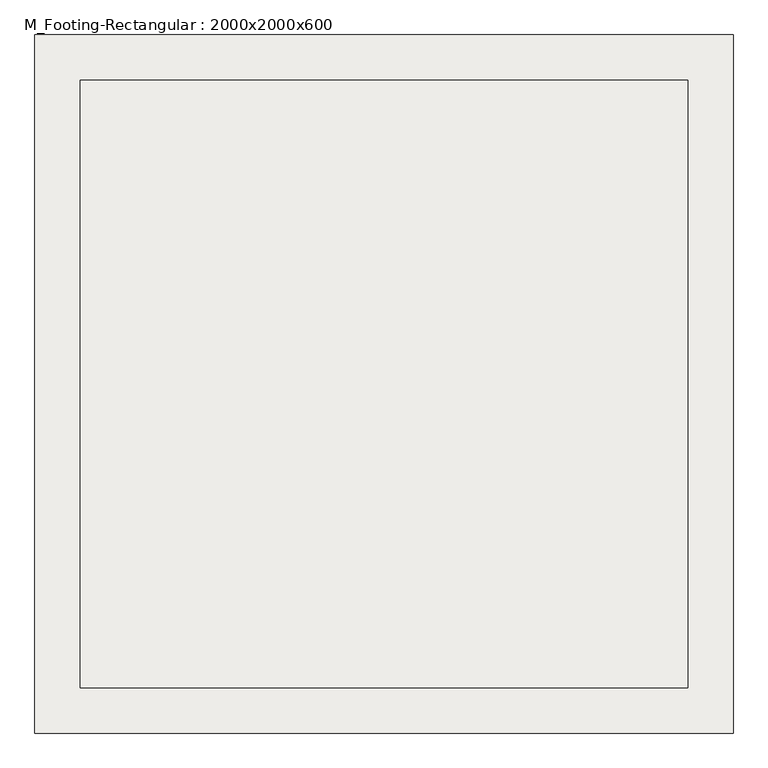
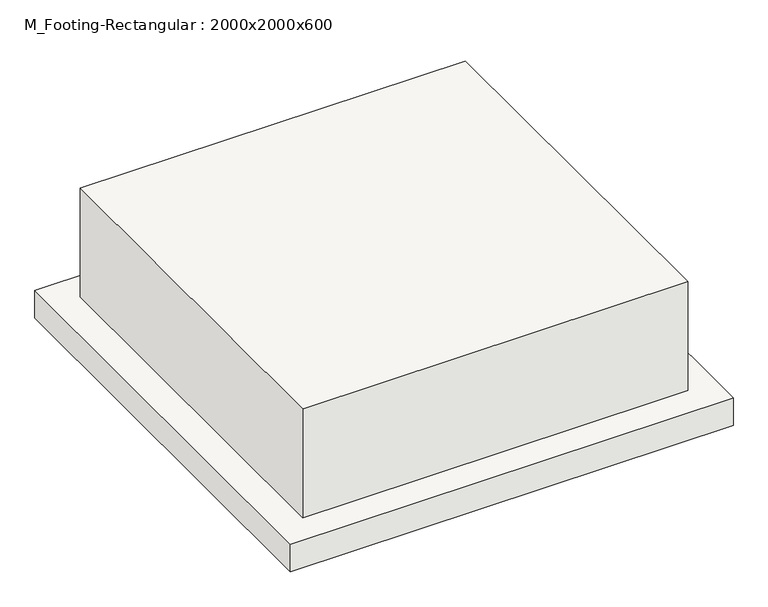
"""IFC4 building model written with IfcOpenShell, lengths in millimetres: slab geometry, M_Footing-Rectangular : 2000x2000x600."""

from ifc_helpers import new_model, si_unit, frame, origin, place, context, project, spatial, polyline, outline, extrude, source, transform, mapped, element, save


def m_footing_rectangular_2000x2000x600_e4767d7a(model_context):
    return source(origin(), model_context, "Body", "SweptSolid", [
        extrude(outline(polyline([(1150.0, 1150.0), (1150.0, -1150.0), (-1150.0, -1150.0), (-1150.0, 1150.0), (1150.0, 1150.0)])), frame((0.0, 0.0, -752.4), z_axis=(0.0, 0.0, 1.0), x_axis=(1.0, 0.0, 0.0)), (0.0, 0.0, 1.0), 152.4),
        extrude(outline(polyline([(1000.0, 1000.0), (1000.0, -1000.0), (-1000.0, -1000.0), (-1000.0, 1000.0), (1000.0, 1000.0)])), frame((0.0, 0.0, -600.0), z_axis=(0.0, 0.0, 1.0), x_axis=(1.0, 0.0, 0.0)), (0.0, 0.0, 1.0), 600.0),
    ])


if __name__ == "__main__":
    model = new_model("IFC4")
    model_context = context("Model", 3, world=origin())
    ifc_project = project(units=[si_unit("LENGTHUNIT", "METRE", prefix="MILLI")], contexts=[model_context])
    site = spatial("IfcSite", under=ifc_project)
    building = spatial("IfcBuilding", under=site)
    placement = place(None, origin())
    m_footing_rectangular_2000x2000x600_shape = m_footing_rectangular_2000x2000x600_e4767d7a(model_context)
    element("IfcSlab", 1, ObjectType="M_Footing-Rectangular : 2000x2000x600", at=placement, inside=building, context=model_context, shape_type="MappedRepresentation", body=[
        mapped(m_footing_rectangular_2000x2000x600_shape, transform((0.0, 0.0, 0.0), x_axis=(1.0, 0.0, 0.0), y_axis=(0.0, 1.0, 0.0), z_axis=(0.0, 0.0, 1.0))),
    ])
    save(model, "model.ifc")

# Revit data of these elements
# Type "M_Footing-Rectangular : 2000x2000x600"
#   Width = 2000 mm
#   Length = 2000 mm
#   Foundation Thickness = 600 mm
#   Structural Material [instance default] = Concrete, Cast-in-Place gray
#   Assembly Code = ""
# Element 1 (IfcSlab, "M_Footing-Rectangular : 2000x2000x600")
#   Materials on its faces: "Concrete, Cast-in-Place gray"
# Materials
#   "Concrete, Cast-in-Place gray": class "Concrete", colour RGB 192 192 192, transparency 0, Description = "Cast-in-place concrete", Cost = 0
